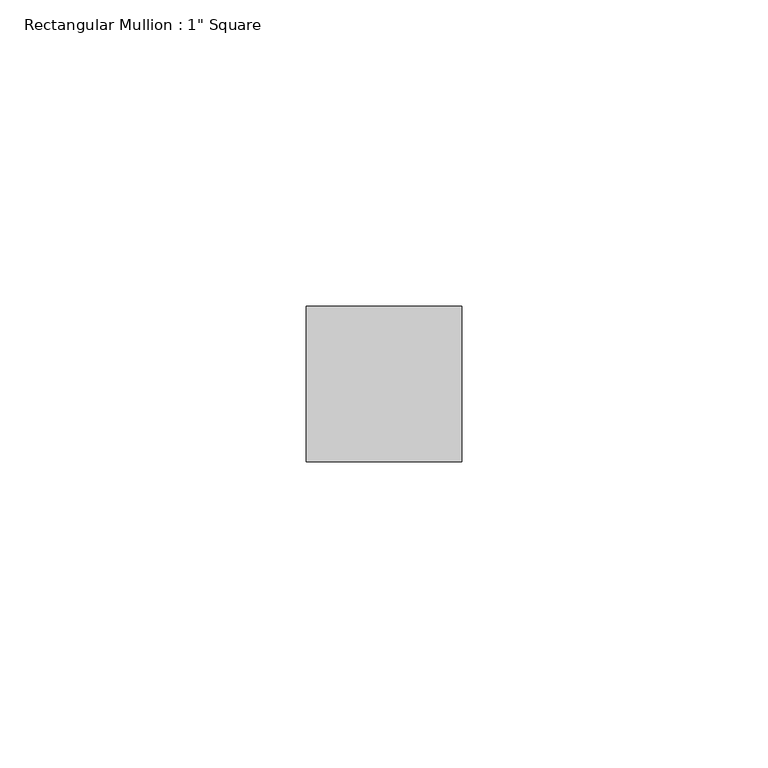
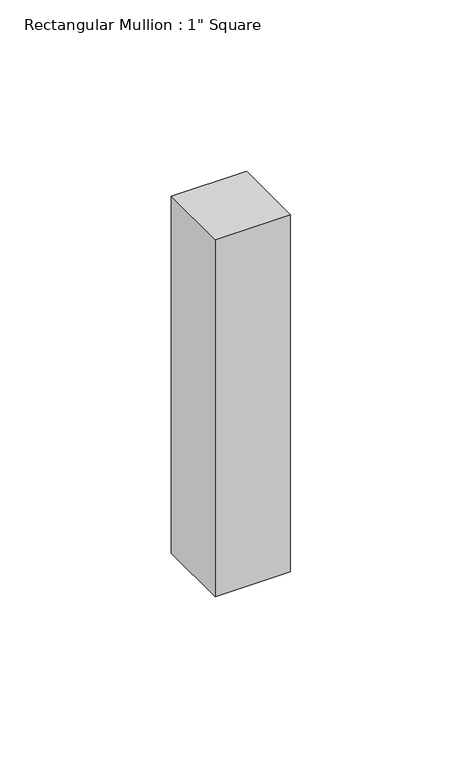
"""IFC4 building model written with IfcOpenShell, lengths in millimetres: member geometry."""

from ifc_helpers import new_model, si_unit, frame, origin, place, context, project, spatial, polyline, outline, extrude, source, transform, mapped, element, save


def member_4ec4fa50(model_context):
    return source(origin(), model_context, "Body", "SweptSolid", [
        extrude(outline(polyline([(0.0, 12.7), (0.0, -12.7), (-25.4, -12.7), (-25.4, 12.7), (0.0, 12.7)])), frame((0.0, 0.0, -127.0), z_axis=(0.0, 0.0, 1.0), x_axis=(1.0, 0.0, 0.0)), (0.0, 0.0, 1.0), 127.0),
    ])


if __name__ == "__main__":
    model = new_model("IFC4")
    model_context = context("Model", 3, world=origin())
    ifc_project = project(units=[si_unit("LENGTHUNIT", "METRE", prefix="MILLI")], contexts=[model_context])
    site = spatial("IfcSite", under=ifc_project)
    building = spatial("IfcBuilding", under=site)
    placement = place(None, origin())
    member_shape = member_4ec4fa50(model_context)
    element("IfcMember", 1, ObjectType="Rectangular Mullion : 1\" Square", at=placement, inside=building, context=model_context, shape_type="MappedRepresentation", body=[
        mapped(member_shape, transform((0.0, 0.0, 0.0), x_axis=(1.0, 0.0, 0.0), y_axis=(0.0, 1.0, 0.0), z_axis=(0.0, 0.0, 1.0))),
    ])
    save(model, "model.ifc")

# Revit data of these elements
# Type "Rectangular Mullion : 1\" Square"
#   built-in parameter 1007304 = 0.0833333 (stored number, unit not read)
#   built-in parameter 1007301 = 0.0416667 (stored number, unit not read)
#   built-in parameter 1007300 = 0.0416667 (stored number, unit not read)
# Element 1 (IfcMember, "Rectangular Mullion : 1\" Square")
#   Materials on its faces: "black"
# Materials
#   "black": class "Generic", colour RGB 120 120 120, transparency 0, Cost = 0
